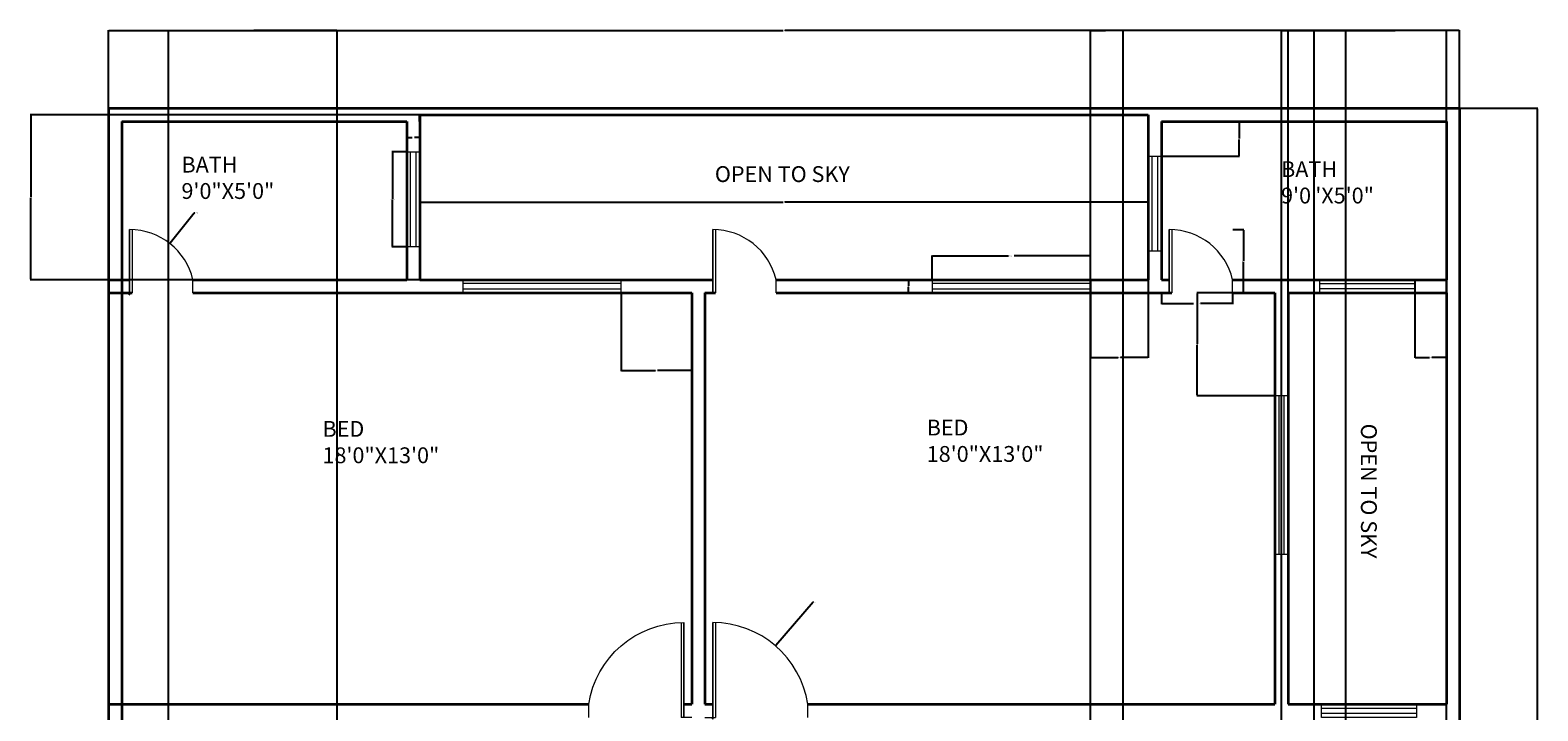
# Model space of a CAD drawing. Units: inches. Extents: x 40921 to 41493, y 89872 to 90511.
# Tile 4 of 4: x 40921 to 41493, y 90253 to 90511. Entities that reach past the tile are written whole.
import ezdxf

# ---------------------------------------------------------------- set-up
doc = ezdxf.new("R2010")
doc.units = ezdxf.units.IN
doc.header["$MEASUREMENT"] = 0
for name, color, linetype, lineweight in [('A-ANNO-DIMS', 2, 'Continuous', 18), ('A-AREA-IDEN', 7, 'Continuous', 18), ('A-DOOR', 3, 'Continuous', 20), ('A-GLAZ', 4, 'Continuous', 18), ('A-WALL', 7, 'Continuous', 35)]:
    doc.layers.add(name, color=color, linetype=linetype, lineweight=lineweight)
doc.styles.get("Standard").update_dxf_attribs({"font": 'arial.ttf'})
doc.dimstyles.get("Standard").update_dxf_attribs({"dimtxt": 0.18, "dimasz": 0.18, "dimexe": 0.18, "dimexo": 0.0625, "dimgap": 0.09, "dimtad": 0, "dimtih": 1, "dimtoh": 1, "dimdec": 4, "dimzin": 0, "dimdsep": 46, "dimtxsty": 'Standard', "dimcen": 0.09, "dimadec": 0, "dimazin": 0, "dimtfac": 1, "dimtdec": 4, "dimtofl": 0, "dimtmove": 0, "dimatfit": 3, "dimfxl": 1, "dimtolj": 1, "dimtzin": 0, "dimarcsym": 0})

# ---------------------------------------------------------------- blocks, each defined once
blk = doc.blocks.new('DOOR-SWING-24IN')
for p, q in [((3, 0), (3, 24)), ((3, 24), (3, 0)), ((4, 24), (4, 0)), ((27, 0), (27, 5)), ((0, 0), (3, 0)), ((3, 0), (4, 0))]:
    blk.add_line(p, q)
blk.add_arc((3, -0.66), 24.66, 13.265, 90)
blk = doc.blocks.new('DOOR-SWING-36IN')
for p, q in [((3, 0), (3, 36)), ((3, 36), (3, 0)), ((4, 36), (4, 0)), ((39, 0), (39, 5)), ((0, 0), (3, 0)), ((3, 0), (4, 0))]:
    blk.add_line(p, q)
blk.add_arc((3, -0.4), 36.4, 8.5358, 90)
blk = doc.blocks.new('WIN-36IN')
for p, q in [((0, 36), (5, 36)), ((0, 0), (0, 36)), ((1.5, 0), (1.5, 36)), ((3.5, 36), (3.5, 0)), ((5, 36), (5, 0)), ((5, 0), (0, 0))]:
    blk.add_line(p, q)
blk = doc.blocks.new('WIN-60IN')
for p, q in [((0, 5), (0, 0)), ((60, 5), (0, 5)), ((60, 3.5), (0, 3.5)), ((0, 1.5), (60, 1.5)), ((60, 0), (60, 5)), ((0, 0), (60, 0))]:
    blk.add_line(p, q)
blk = doc.blocks.new('*D7')
at = {"layer": 'A-ANNO-DIMS', "color": 0, "lineweight": -2, "transparency": 16777216}
for p, q in [((41064.09, 90465.09), (41058.57, 90465.09)), ((41058.75, 90464.91), (41058.75, 90447.27)), ((41058.75, 90429.27), (41058.75, 90446.9)), ((41064.09, 90429.09), (41058.57, 90429.09))]:
    blk.add_line(p, q, dxfattribs=at)
at = {"layer": 'A-ANNO-DIMS', "color": 0, "transparency": 16777216}
for points in [[(41058.72, 90464.91), (41058.78, 90464.91), (41058.75, 90465.09)], [(41058.72, 90429.27), (41058.78, 90429.27), (41058.75, 90429.09)]]:
    blk.add_solid(points, dxfattribs=at)
at = {"layer": 'Defpoints', "color": 0, "transparency": 16777216}
for p in [(41058.75, 90465.09), (41064.15, 90465.09), (41064.15, 90429.09)]:
    blk.add_point(p, dxfattribs=at)
at = {"layer": 'A-ANNO-DIMS', "color": 0, "transparency": 16777216, "insert": (41058.75, 90447.09), "char_height": 0.18, "attachment_point": 5}
blk.add_mtext('\\A1;WINDOW 36 TYP.', dxfattribs=at)
blk = doc.blocks.new('*D8')
at = {"layer": 'A-ANNO-DIMS', "color": 0, "lineweight": -2, "transparency": 16777216}
for p, q in [((41064.15, 90465.15), (41064.15, 90470.67)), ((41064.33, 90470.49), (41066.19, 90470.49)), ((41068.97, 90470.49), (41067.11, 90470.49)), ((41069.15, 90465.15), (41069.15, 90470.67))]:
    blk.add_line(p, q, dxfattribs=at)
at = {"layer": 'A-ANNO-DIMS', "color": 0, "transparency": 16777216}
for points in [[(41064.33, 90470.52), (41064.33, 90470.46), (41064.15, 90470.49)], [(41068.97, 90470.52), (41068.97, 90470.46), (41069.15, 90470.49)]]:
    blk.add_solid(points, dxfattribs=at)
at = {"layer": 'Defpoints', "color": 0, "transparency": 16777216}
for p in [(41069.15, 90470.49), (41064.15, 90465.09), (41069.15, 90465.09)]:
    blk.add_point(p, dxfattribs=at)
at = {"layer": 'A-ANNO-DIMS', "color": 0, "transparency": 16777216, "insert": (41066.65, 90470.49), "char_height": 0.18, "attachment_point": 5}
blk.add_mtext('\\A1;5 TYP.', dxfattribs=at)
blk = doc.blocks.new('*D9')
at = {"layer": 'A-ANNO-DIMS', "color": 0, "lineweight": -2, "transparency": 16777216}
for p, q in [((41263.29, 90416.69), (41263.29, 90425.81)), ((41263.47, 90425.63), (41292.18, 90425.63)), ((41323.11, 90425.63), (41294.41, 90425.63)), ((41323.29, 90416.69), (41323.29, 90425.81))]:
    blk.add_line(p, q, dxfattribs=at)
at = {"layer": 'A-ANNO-DIMS', "color": 0, "transparency": 16777216}
for points in [[(41263.47, 90425.66), (41263.47, 90425.6), (41263.29, 90425.63)], [(41323.11, 90425.66), (41323.11, 90425.6), (41323.29, 90425.63)]]:
    blk.add_solid(points, dxfattribs=at)
at = {"layer": 'Defpoints', "color": 0, "transparency": 16777216}
for p in [(41263.29, 90425.63), (41263.29, 90416.63), (41323.29, 90416.63)]:
    blk.add_point(p, dxfattribs=at)
at = {"layer": 'A-ANNO-DIMS', "color": 0, "transparency": 16777216, "insert": (41293.29, 90425.63), "char_height": 0.18, "attachment_point": 5}
blk.add_mtext('\\A1;WINDOW 60 TYP.', dxfattribs=at)
blk = doc.blocks.new('*D10')
at = {"layer": 'A-ANNO-DIMS', "color": 0, "lineweight": -2, "transparency": 16777216}
for p, q in [((41263.23, 90416.63), (41254.11, 90416.63)), ((41254.29, 90416.45), (41254.29, 90414.31)), ((41263.23, 90411.63), (41254.11, 90411.63)), ((41254.29, 90411.81), (41254.29, 90413.95))]:
    blk.add_line(p, q, dxfattribs=at)
at = {"layer": 'A-ANNO-DIMS', "color": 0, "transparency": 16777216}
for points in [[(41254.26, 90416.45), (41254.32, 90416.45), (41254.29, 90416.63)], [(41254.26, 90411.81), (41254.32, 90411.81), (41254.29, 90411.63)]]:
    blk.add_solid(points, dxfattribs=at)
at = {"layer": 'Defpoints', "color": 0, "transparency": 16777216}
for p in [(41263.29, 90416.63), (41254.29, 90411.63), (41263.29, 90411.63)]:
    blk.add_point(p, dxfattribs=at)
at = {"layer": 'A-ANNO-DIMS', "color": 0, "transparency": 16777216, "insert": (41254.29, 90414.13), "char_height": 0.18, "attachment_point": 5}
blk.add_mtext('\\A1;5 TYP.', dxfattribs=at)
blk = doc.blocks.new('*D13')
at = {"layer": 'A-ANNO-DIMS', "color": 0, "lineweight": -2, "transparency": 16777216}
for p, q in [((41350.15, 90411.57), (41350.15, 90407.4)), ((41377.15, 90411.57), (41377.15, 90407.4)), ((41350.33, 90407.58), (41362.34, 90407.58)), ((41376.97, 90407.58), (41364.96, 90407.58))]:
    blk.add_line(p, q, dxfattribs=at)
at = {"layer": 'A-ANNO-DIMS', "color": 0, "transparency": 16777216}
for points in [[(41350.33, 90407.61), (41350.33, 90407.55), (41350.15, 90407.58)], [(41376.97, 90407.61), (41376.97, 90407.55), (41377.15, 90407.58)]]:
    blk.add_solid(points, dxfattribs=at)
at = {"layer": 'Defpoints', "color": 0, "transparency": 16777216}
for p in [(41350.15, 90411.63), (41377.15, 90411.63), (41377.15, 90407.58)]:
    blk.add_point(p, dxfattribs=at)
at = {"layer": 'A-ANNO-DIMS', "color": 0, "transparency": 16777216, "insert": (41363.65, 90407.58), "char_height": 0.18, "attachment_point": 5}
blk.add_mtext('\\A1;BATH DOOR 27 TYP.', dxfattribs=at)
blk = doc.blocks.new('*D14')
at = {"layer": 'A-ANNO-DIMS', "color": 0, "lineweight": -2, "transparency": 16777216}
for p, q in [((41377.21, 90435.63), (41381.38, 90435.63)), ((41381.2, 90435.45), (41381.2, 90423.81)), ((41381.2, 90411.81), (41381.2, 90423.45)), ((41377.21, 90411.63), (41381.38, 90411.63))]:
    blk.add_line(p, q, dxfattribs=at)
at = {"layer": 'A-ANNO-DIMS', "color": 0, "transparency": 16777216}
for points in [[(41381.17, 90435.45), (41381.23, 90435.45), (41381.2, 90435.63)], [(41381.17, 90411.81), (41381.23, 90411.81), (41381.2, 90411.63)]]:
    blk.add_solid(points, dxfattribs=at)
at = {"layer": 'Defpoints', "color": 0, "transparency": 16777216}
for p in [(41377.15, 90435.63), (41381.2, 90435.63), (41377.15, 90411.63)]:
    blk.add_point(p, dxfattribs=at)
at = {"layer": 'A-ANNO-DIMS', "color": 0, "transparency": 16777216, "insert": (41381.2, 90423.63), "char_height": 0.18, "attachment_point": 5}
blk.add_mtext('\\A1;24 TYP.', dxfattribs=at)
blk = doc.blocks.new('*D19')
at = {"layer": 'A-ANNO-DIMS', "color": 0, "lineweight": -2, "transparency": 16777216}
for p, q in [((40951.15, 90481.69), (40951.15, 90511.26)), ((40951.33, 90511.08), (41206.86, 90511.08)), ((41462.97, 90511.08), (41207.44, 90511.08)), ((41463.15, 90481.69), (41463.15, 90511.26))]:
    blk.add_line(p, q, dxfattribs=at)
at = {"layer": 'A-ANNO-DIMS', "color": 0, "transparency": 16777216}
for points in [[(40951.33, 90511.11), (40951.33, 90511.05), (40951.15, 90511.08)], [(41462.97, 90511.11), (41462.97, 90511.05), (41463.15, 90511.08)]]:
    blk.add_solid(points, dxfattribs=at)
at = {"layer": 'Defpoints', "color": 0, "transparency": 16777216}
for p in [(41463.15, 90511.08), (40951.15, 90481.63), (41463.15, 90481.63)]:
    blk.add_point(p, dxfattribs=at)
at = {"layer": 'A-ANNO-DIMS', "color": 0, "transparency": 16777216, "insert": (41207.15, 90511.08), "char_height": 0.18, "attachment_point": 5}
blk.add_mtext('\\A1;512', dxfattribs=at)
blk = doc.blocks.new('*D20')
at = {"layer": 'A-ANNO-DIMS', "color": 0, "lineweight": -2, "transparency": 16777216}
for p, q in [((41463.21, 90481.63), (41492.78, 90481.63)), ((41492.6, 90481.45), (41492.6, 90191.81)), ((41492.6, 89901.81), (41492.6, 90191.45)), ((41463.21, 89901.63), (41492.78, 89901.63))]:
    blk.add_line(p, q, dxfattribs=at)
at = {"layer": 'A-ANNO-DIMS', "color": 0, "transparency": 16777216}
for points in [[(41492.57, 90481.45), (41492.63, 90481.45), (41492.6, 90481.63)], [(41492.57, 89901.81), (41492.63, 89901.81), (41492.6, 89901.63)]]:
    blk.add_solid(points, dxfattribs=at)
at = {"layer": 'Defpoints', "color": 0, "transparency": 16777216}
for p in [(41463.15, 90481.63), (41492.6, 90481.63), (41463.15, 89901.63)]:
    blk.add_point(p, dxfattribs=at)
at = {"layer": 'A-ANNO-DIMS', "color": 0, "transparency": 16777216, "insert": (41492.6, 90191.63), "char_height": 0.18, "attachment_point": 5}
blk.add_mtext('\\A1;580', dxfattribs=at)
blk = doc.blocks.new('*D21')
at = {"layer": 'A-ANNO-DIMS', "color": 0, "lineweight": -2, "transparency": 16777216}
for p, q in [((41069.15, 90416.69), (41069.15, 90446.26)), ((41069.33, 90446.08), (41206.86, 90446.08)), ((41344.97, 90446.08), (41207.44, 90446.08)), ((41345.15, 90416.69), (41345.15, 90446.26))]:
    blk.add_line(p, q, dxfattribs=at)
at = {"layer": 'A-ANNO-DIMS', "color": 0, "transparency": 16777216}
for points in [[(41069.33, 90446.11), (41069.33, 90446.05), (41069.15, 90446.08)], [(41344.97, 90446.11), (41344.97, 90446.05), (41345.15, 90446.08)]]:
    blk.add_solid(points, dxfattribs=at)
at = {"layer": 'Defpoints', "color": 0, "transparency": 16777216}
for p in [(41345.15, 90446.08), (41069.15, 90416.63), (41345.15, 90416.63)]:
    blk.add_point(p, dxfattribs=at)
at = {"layer": 'A-ANNO-DIMS', "color": 0, "transparency": 16777216, "insert": (41207.15, 90446.08), "char_height": 0.18, "attachment_point": 5}
blk.add_mtext('\\A1;276', dxfattribs=at)
blk = doc.blocks.new('*D22')
at = {"layer": 'A-ANNO-DIMS', "color": 0, "lineweight": -2, "transparency": 16777216}
for p, q in [((41069.09, 90479.13), (40921.52, 90479.13)), ((40921.7, 90478.95), (40921.7, 90448.06)), ((40921.7, 90416.81), (40921.7, 90447.7)), ((41069.09, 90416.63), (40921.52, 90416.63))]:
    blk.add_line(p, q, dxfattribs=at)
at = {"layer": 'A-ANNO-DIMS', "color": 0, "transparency": 16777216}
for points in [[(40921.67, 90478.95), (40921.73, 90478.95), (40921.7, 90479.13)], [(40921.67, 90416.81), (40921.73, 90416.81), (40921.7, 90416.63)]]:
    blk.add_solid(points, dxfattribs=at)
at = {"layer": 'Defpoints', "color": 0, "transparency": 16777216}
for p in [(41069.15, 90479.13), (40921.7, 90416.63), (41069.15, 90416.63)]:
    blk.add_point(p, dxfattribs=at)
at = {"layer": 'A-ANNO-DIMS', "color": 0, "transparency": 16777216, "insert": (40921.7, 90447.88), "char_height": 0.18, "attachment_point": 5}
blk.add_mtext('\\A1;62.5', dxfattribs=at)
blk = doc.blocks.new('*D23')
at = {"layer": 'A-ANNO-DIMS', "color": 0, "lineweight": -2, "transparency": 16777216}
for p, q in [((41398.15, 90255.69), (41398.15, 90511.26)), ((41398.33, 90511.08), (41427.93, 90511.08)), ((41457.97, 90511.08), (41428.37, 90511.08)), ((41458.15, 90255.69), (41458.15, 90511.26))]:
    blk.add_line(p, q, dxfattribs=at)
at = {"layer": 'A-ANNO-DIMS', "color": 0, "transparency": 16777216}
for points in [[(41398.33, 90511.11), (41398.33, 90511.05), (41398.15, 90511.08)], [(41457.97, 90511.11), (41457.97, 90511.05), (41458.15, 90511.08)]]:
    blk.add_solid(points, dxfattribs=at)
at = {"layer": 'Defpoints', "color": 0, "transparency": 16777216}
for p in [(41458.15, 90511.08), (41398.15, 90255.63), (41458.15, 90255.63)]:
    blk.add_point(p, dxfattribs=at)
at = {"layer": 'A-ANNO-DIMS', "color": 0, "transparency": 16777216, "insert": (41428.15, 90511.08), "char_height": 0.18, "attachment_point": 5}
blk.add_mtext('\\A1;60', dxfattribs=at)
blk = doc.blocks.new('*D25')
at = {"layer": 'A-ANNO-DIMS', "color": 0, "lineweight": -2, "transparency": 16777216}
for p, q in [((40973.9, 90106.69), (40973.9, 90511.26)), ((40974.08, 90511.08), (41005.48, 90511.08)), ((41037.63, 90511.08), (41006.23, 90511.08)), ((41037.81, 90106.69), (41037.81, 90511.26))]:
    blk.add_line(p, q, dxfattribs=at)
at = {"layer": 'A-ANNO-DIMS', "color": 0, "transparency": 16777216}
for points in [[(40974.08, 90511.11), (40974.08, 90511.05), (40973.9, 90511.08)], [(41037.63, 90511.11), (41037.63, 90511.05), (41037.81, 90511.08)]]:
    blk.add_solid(points, dxfattribs=at)
at = {"layer": 'Defpoints', "color": 0, "transparency": 16777216}
for p in [(41037.81, 90511.08), (40973.9, 90106.63), (41037.81, 90106.63)]:
    blk.add_point(p, dxfattribs=at)
at = {"layer": 'A-ANNO-DIMS', "color": 0, "transparency": 16777216, "insert": (41005.85, 90511.08), "char_height": 0.18, "attachment_point": 5}
blk.add_mtext('\\A1;63.91', dxfattribs=at)
blk = doc.blocks.new('*D31')
at = {"layer": 'A-ANNO-DIMS', "color": 0, "lineweight": -2, "transparency": 16777216}
for p, q in [((41420.03, 89906.69), (41420.03, 90511.26)), ((41420.21, 90511.08), (41438.7, 90511.08)), ((41457.97, 90511.08), (41439.48, 90511.08)), ((41458.15, 89906.69), (41458.15, 90511.26))]:
    blk.add_line(p, q, dxfattribs=at)
at = {"layer": 'A-ANNO-DIMS', "color": 0, "transparency": 16777216}
for points in [[(41420.21, 90511.11), (41420.21, 90511.05), (41420.03, 90511.08)], [(41457.97, 90511.11), (41457.97, 90511.05), (41458.15, 90511.08)]]:
    blk.add_solid(points, dxfattribs=at)
at = {"layer": 'Defpoints', "color": 0, "transparency": 16777216}
for p in [(41458.15, 90511.08), (41420.03, 89906.63), (41458.15, 89906.63)]:
    blk.add_point(p, dxfattribs=at)
at = {"layer": 'A-ANNO-DIMS', "color": 0, "transparency": 16777216, "insert": (41439.09, 90511.08), "char_height": 0.18, "attachment_point": 5}
blk.add_mtext('\\A1;38.12', dxfattribs=at)
blk = doc.blocks.new('*D32')
at = {"layer": 'A-ANNO-DIMS', "color": 0, "lineweight": -2, "transparency": 16777216}
for p, q in [((41323.33, 89906.69), (41323.33, 90511.26)), ((41323.51, 90511.08), (41329.01, 90511.08)), ((41335.42, 90511.08), (41329.92, 90511.08)), ((41335.6, 89906.69), (41335.6, 90511.26))]:
    blk.add_line(p, q, dxfattribs=at)
at = {"layer": 'A-ANNO-DIMS', "color": 0, "transparency": 16777216}
for points in [[(41323.51, 90511.11), (41323.51, 90511.05), (41323.33, 90511.08)], [(41335.42, 90511.11), (41335.42, 90511.05), (41335.6, 90511.08)]]:
    blk.add_solid(points, dxfattribs=at)
at = {"layer": 'Defpoints', "color": 0, "transparency": 16777216}
for p in [(41335.6, 90511.08), (41323.33, 89906.63), (41335.6, 89906.63)]:
    blk.add_point(p, dxfattribs=at)
at = {"layer": 'A-ANNO-DIMS', "color": 0, "transparency": 16777216, "insert": (41329.46, 90511.08), "char_height": 0.18, "attachment_point": 5}
blk.add_mtext('\\A1;12.272', dxfattribs=at)
blk = doc.blocks.new('*D33')
at = {"layer": 'A-ANNO-DIMS', "color": 0, "lineweight": -2, "transparency": 16777216}
for p, q in [((41395.6, 89906.69), (41395.6, 90511.26)), ((41395.78, 90511.08), (41401.36, 90511.08)), ((41407.85, 90511.08), (41402.27, 90511.08)), ((41408.03, 89906.69), (41408.03, 90511.26))]:
    blk.add_line(p, q, dxfattribs=at)
at = {"layer": 'A-ANNO-DIMS', "color": 0, "transparency": 16777216}
for points in [[(41395.78, 90511.11), (41395.78, 90511.05), (41395.6, 90511.08)], [(41407.85, 90511.11), (41407.85, 90511.05), (41408.03, 90511.08)]]:
    blk.add_solid(points, dxfattribs=at)
at = {"layer": 'Defpoints', "color": 0, "transparency": 16777216}
for p in [(41408.03, 90511.08), (41395.6, 89906.63), (41408.03, 89906.63)]:
    blk.add_point(p, dxfattribs=at)
at = {"layer": 'A-ANNO-DIMS', "color": 0, "transparency": 16777216, "insert": (41401.81, 90511.08), "char_height": 0.18, "attachment_point": 5}
blk.add_mtext('\\A1;12.429', dxfattribs=at)
blk = doc.blocks.new('*D36')
at = {"layer": 'A-ANNO-DIMS', "color": 0, "lineweight": -2, "transparency": 16777216}
for p, q in [((41145.4, 90411.57), (41145.4, 90382)), ((41172.15, 90411.57), (41172.15, 90382)), ((41145.58, 90382.18), (41158.38, 90382.18)), ((41171.97, 90382.18), (41159.17, 90382.18))]:
    blk.add_line(p, q, dxfattribs=at)
at = {"layer": 'A-ANNO-DIMS', "color": 0, "transparency": 16777216}
for points in [[(41145.58, 90382.21), (41145.58, 90382.15), (41145.4, 90382.18)], [(41171.97, 90382.21), (41171.97, 90382.15), (41172.15, 90382.18)]]:
    blk.add_solid(points, dxfattribs=at)
at = {"layer": 'Defpoints', "color": 0, "transparency": 16777216}
for p in [(41145.4, 90411.63), (41172.15, 90411.63), (41145.4, 90382.18)]:
    blk.add_point(p, dxfattribs=at)
at = {"layer": 'A-ANNO-DIMS', "color": 0, "transparency": 16777216, "insert": (41158.77, 90382.18), "char_height": 0.18, "attachment_point": 5}
blk.add_mtext('\\A1;26.75', dxfattribs=at)
blk = doc.blocks.new('*D37')
at = {"layer": 'A-ANNO-DIMS', "color": 0, "lineweight": -2, "transparency": 16777216}
for p, q in [((41323.29, 90416.57), (41323.29, 90387)), ((41345.15, 90416.57), (41345.15, 90387)), ((41323.47, 90387.18), (41333.76, 90387.18)), ((41344.97, 90387.18), (41334.69, 90387.18))]:
    blk.add_line(p, q, dxfattribs=at)
at = {"layer": 'A-ANNO-DIMS', "color": 0, "transparency": 16777216}
for points in [[(41323.47, 90387.21), (41323.47, 90387.15), (41323.29, 90387.18)], [(41344.97, 90387.21), (41344.97, 90387.15), (41345.15, 90387.18)]]:
    blk.add_solid(points, dxfattribs=at)
at = {"layer": 'Defpoints', "color": 0, "transparency": 16777216}
for p in [(41323.29, 90416.63), (41345.15, 90416.63), (41323.29, 90387.18)]:
    blk.add_point(p, dxfattribs=at)
at = {"layer": 'A-ANNO-DIMS', "color": 0, "transparency": 16777216, "insert": (41334.22, 90387.18), "char_height": 0.18, "attachment_point": 5}
blk.add_mtext('\\A1;21.857', dxfattribs=at)
blk = doc.blocks.new('*D38')
at = {"layer": 'A-ANNO-DIMS', "color": 0, "lineweight": -2, "transparency": 16777216}
for p, q in [((41393.09, 90411.63), (41363.52, 90411.63)), ((41363.7, 90411.45), (41363.7, 90392.3)), ((41363.7, 90372.79), (41363.7, 90391.94)), ((41393.09, 90372.61), (41363.52, 90372.61))]:
    blk.add_line(p, q, dxfattribs=at)
at = {"layer": 'A-ANNO-DIMS', "color": 0, "transparency": 16777216}
for points in [[(41363.67, 90411.45), (41363.73, 90411.45), (41363.7, 90411.63)], [(41363.67, 90372.79), (41363.73, 90372.79), (41363.7, 90372.61)]]:
    blk.add_solid(points, dxfattribs=at)
at = {"layer": 'Defpoints', "color": 0, "transparency": 16777216}
for p in [(41363.7, 90411.63), (41393.15, 90411.63), (41393.15, 90372.61)]:
    blk.add_point(p, dxfattribs=at)
at = {"layer": 'A-ANNO-DIMS', "color": 0, "transparency": 16777216, "insert": (41363.7, 90392.12), "char_height": 0.18, "attachment_point": 5}
blk.add_mtext('\\A1;39.02', dxfattribs=at)
blk = doc.blocks.new('*D39')
at = {"layer": 'A-ANNO-DIMS', "color": 0, "lineweight": -2, "transparency": 16777216}
for p, q in [((41446.17, 90416.57), (41446.17, 90387)), ((41458.15, 90416.57), (41458.15, 90387)), ((41446.35, 90387.18), (41451.7, 90387.18)), ((41457.97, 90387.18), (41452.61, 90387.18))]:
    blk.add_line(p, q, dxfattribs=at)
at = {"layer": 'A-ANNO-DIMS', "color": 0, "transparency": 16777216}
for points in [[(41446.35, 90387.21), (41446.35, 90387.15), (41446.17, 90387.18)], [(41457.97, 90387.21), (41457.97, 90387.15), (41458.15, 90387.18)]]:
    blk.add_solid(points, dxfattribs=at)
at = {"layer": 'Defpoints', "color": 0, "transparency": 16777216}
for p in [(41446.17, 90416.63), (41458.15, 90416.63), (41446.17, 90387.18)]:
    blk.add_point(p, dxfattribs=at)
at = {"layer": 'A-ANNO-DIMS', "color": 0, "transparency": 16777216, "insert": (41452.16, 90387.18), "char_height": 0.18, "attachment_point": 5}
blk.add_mtext('\\A1;11.983', dxfattribs=at)
blk = doc.blocks.new('*D45')
at = {"layer": 'A-ANNO-DIMS', "color": 0, "lineweight": -2, "transparency": 16777216}
for p, q in [((41350.21, 90476.63), (41379.78, 90476.63)), ((41379.6, 90476.45), (41379.6, 90470.21)), ((41379.6, 90463.61), (41379.6, 90469.85)), ((41350.21, 90463.43), (41379.78, 90463.43))]:
    blk.add_line(p, q, dxfattribs=at)
at = {"layer": 'A-ANNO-DIMS', "color": 0, "transparency": 16777216}
for points in [[(41379.57, 90476.45), (41379.63, 90476.45), (41379.6, 90476.63)], [(41379.57, 90463.61), (41379.63, 90463.61), (41379.6, 90463.43)]]:
    blk.add_solid(points, dxfattribs=at)
at = {"layer": 'Defpoints', "color": 0, "transparency": 16777216}
for p in [(41350.15, 90476.63), (41350.15, 90463.43), (41379.6, 90463.43)]:
    blk.add_point(p, dxfattribs=at)
at = {"layer": 'A-ANNO-DIMS', "color": 0, "transparency": 16777216, "insert": (41379.6, 90470.03), "char_height": 0.18, "attachment_point": 5}
blk.add_mtext('\\A1;13.197', dxfattribs=at)
blk = doc.blocks.new('*D46')
at = {"layer": 'A-ANNO-DIMS', "color": 0, "lineweight": -2, "transparency": 16777216}
for p, q in [((41218.16, 90294.36), (41204.02, 90277.95)), ((41218.34, 90294.36), (41218.16, 90294.36)), ((41180.06, 90250.23), (41180.24, 90250.23)), ((41180.15, 90250.14), (41180.15, 90250.32))]:
    blk.add_line(p, q, dxfattribs=at)
at = {"layer": 'A-ANNO-DIMS', "color": 0, "transparency": 16777216}
blk.add_solid([(41204, 90277.97), (41204.04, 90277.93), (41203.9, 90277.81)], dxfattribs=at)
at = {"layer": 'Defpoints', "color": 0, "transparency": 16777216}
for p in [(41203.9, 90277.81), (41180.15, 90250.23)]:
    blk.add_point(p, dxfattribs=at)
at = {"layer": 'A-ANNO-DIMS', "color": 0, "transparency": 16777216, "insert": (41218.94, 90294.36), "char_height": 0.18, "attachment_point": 5}
blk.add_mtext('\\A1;2X R36.4', dxfattribs=at)
blk = doc.blocks.new('*D47')
at = {"layer": 'A-ANNO-DIMS', "color": 0, "lineweight": -2, "transparency": 16777216}
for p, q in [((40983.64, 90441.91), (40974.57, 90430.45)), ((40983.82, 90441.91), (40983.64, 90441.91)), ((40959.06, 90410.97), (40959.24, 90410.97)), ((40959.15, 90410.88), (40959.15, 90411.06))]:
    blk.add_line(p, q, dxfattribs=at)
at = {"layer": 'A-ANNO-DIMS', "color": 0, "transparency": 16777216}
blk.add_solid([(40974.54, 90430.47), (40974.59, 90430.43), (40974.46, 90430.31)], dxfattribs=at)
at = {"layer": 'Defpoints', "color": 0, "transparency": 16777216}
for p in [(40974.46, 90430.31), (40959.15, 90410.97)]:
    blk.add_point(p, dxfattribs=at)
at = {"layer": 'A-ANNO-DIMS', "color": 0, "transparency": 16777216, "insert": (40984.49, 90441.91), "char_height": 0.18, "attachment_point": 5}
blk.add_mtext('\\A1;5X R24.66', dxfattribs=at)

msp = doc.modelspace()

# ---------------------------------------------------------------- linework, layer by layer
at = {"layer": 'A-GLAZ'}
for p, q in [((41064.1503, 90465.0876), (41064.1503, 90465.0876)), ((41446.167, 90416.6306), (41446.167, 90416.6306))]:
    msp.add_line(p, q, dxfattribs=at)
at = {"layer": 'A-WALL'}
for p, q in [((40951.1503, 90481.6306), (41463.1503, 90481.6306)), ((40951.1503, 90481.6306), (40951.1503, 89901.6306)), ((41069.1503, 90479.1306), (41069.1503, 90416.6306)), ((41069.1503, 90479.1306), (41069.1503, 90476.6306)), ((41069.1503, 90476.6306), (41069.1503, 90479.1306)), ((41069.1503, 90479.1306), (41345.1503, 90479.1306)), ((41345.1503, 90479.1306), (41345.1503, 90416.6306)), ((41463.1503, 90481.6306), (41463.1503, 89901.6306)), ((40956.1503, 90476.6306), (40956.1503, 90106.6306)), ((40956.1503, 90476.6306), (41064.1503, 90476.6306)), ((41064.1503, 90476.6306), (41064.1503, 90416.6306)), ((41350.1503, 90476.6306), (41350.1503, 90416.6306)), ((41350.1503, 90476.6306), (41458.1503, 90476.6306)), ((41458.1503, 90476.6306), (41458.1503, 90416.6306)), ((40951.1503, 90416.6306), (40959.1503, 90416.6306)), ((40983.1503, 90416.6306), (41064.1503, 90416.6306)), ((41069.1503, 90416.6306), (41180.1503, 90416.6306)), ((41204.1503, 90416.6306), (41345.1503, 90416.6306)), ((41350.1503, 90416.6306), (41353.1503, 90416.6306)), ((41377.1503, 90416.6306), (41458.1503, 90416.6306)), ((40951.1503, 90411.6306), (40960.1503, 90411.6306)), ((40983.1503, 90411.6306), (41172.1503, 90411.6306)), ((41172.1503, 90411.6306), (41172.1503, 90255.6306)), ((41177.1503, 90411.6306), (41177.1503, 90255.6306)), ((41177.1503, 90411.6306), (41181.1503, 90411.6306)), ((41204.1503, 90411.6306), (41354.1503, 90411.6306)), ((41377.1503, 90411.6306), (41393.1503, 90411.6306)), ((41393.1503, 90411.6306), (41393.1503, 90255.6306)), ((41398.1503, 90411.6306), (41398.1503, 90255.6306)), ((41398.1503, 90411.6306), (41458.1503, 90411.6306)), ((41458.1503, 90411.6306), (41458.1503, 90255.6306)), ((40951.1503, 90255.6306), (41133.1503, 90255.6306)), ((41169.1503, 90255.6306), (41172.1503, 90255.6306)), ((41177.1503, 90255.6306), (41180.1503, 90255.6306)), ((41216.1503, 90255.6306), (41393.1503, 90255.6306)), ((41398.1503, 90255.6306), (41458.1503, 90255.6306))]:
    msp.add_line(p, q, dxfattribs=at)

# ---------------------------------------------------------------- block references
at = {"layer": 'A-DOOR'}
for name, p in [('DOOR-SWING-24IN', (40956.15, 90411.631)), ('DOOR-SWING-24IN', (41177.15, 90411.631)), ('DOOR-SWING-24IN', (41350.15, 90411.631)), ('DOOR-SWING-36IN', (41177.15, 90250.631))]:
    msp.add_blockref(name, p, dxfattribs=at)
at = {"layer": 'A-DOOR', "extrusion": (0, 0, -1), "zscale": -1}
msp.add_blockref('DOOR-SWING-36IN', (-41172.1506, 90250.631), dxfattribs=at)
at = {"layer": 'A-GLAZ'}
for name, p in [('WIN-36IN', (41064.15, 90429.088)), ('WIN-36IN', (41345.15, 90427.434)), ('WIN-60IN', (41085.398, 90411.631))]:
    msp.add_blockref(name, p, dxfattribs=at)
for name, p, rotation in [('WIN-60IN', (41323.2934, 90416.6303), 180), ('WIN-36IN', (41446.1666, 90411.6303), 90.00000000000003), ('WIN-60IN', (41393.1507, 90372.6125), 269.9999999999988), ('WIN-36IN', (41446.8101, 90250.6303), 89.99999999999685)]:
    msp.add_blockref(name, p, dxfattribs=dict(at, rotation=rotation))

# ---------------------------------------------------------------- texts
at = {"layer": 'A-AREA-IDEN', "char_height": 6, "attachment_point": 1}
for s, width, insert in [('BATH\\P9\'0"X5\'0"', 65.892116, (40978.8038, 90463.2623)), ('BATH\\P9\'0"X5\'0"', 65.892116, (41395.5067, 90461.5403)), ('OPEN TO SKY', 111.644025, (41180.9345, 90459.6692)), ('BED\\P18\'0"X13\'0"', 70.467307, (41032.2403, 90363.0531)), ('BED\\P18\'0"X13\'0"', 70.467307, (41261.2097, 90363.5572))]:
    msp.add_mtext_dynamic_manual_height_columns(s, width=width, gutter_width=1, heights=[0], dxfattribs=dict(at, insert=insert))
at = {"layer": 'A-AREA-IDEN', "insert": (41431.7814, 90362.0468), "char_height": 6, "attachment_point": 1, "rotation": 270}
msp.add_mtext_dynamic_manual_height_columns('OPEN TO SKY', width=111.644025, gutter_width=1, heights=[0], dxfattribs=at)

# ---------------------------------------------------------------- dimensions: what is measured, and where the dimension line sits
at = {"layer": 'A-ANNO-DIMS'}
for base, p1, p2, override, picture, middle in [((41463.1503, 90511.0806), (40951.1503, 90481.6306), (41463.1503, 90481.6306), {"dimdec": 0, "dimlfac": 1, "dimrnd": 0, "dimzin": 0, "dimdsep": 46, "dimlunit": 2}, '*D19', (41207.1503, 90511.0806)), ((41037.8072, 90511.0806), (40973.8989, 90106.6306), (41037.8072, 90106.6306), {"dimdec": 2, "dimlfac": 1, "dimrnd": 0, "dimzin": 0, "dimdsep": 46, "dimlunit": 2}, '*D25', (41005.8531, 90511.0806)), ((41335.5998, 90511.0806), (41323.3274, 89906.6306), (41335.5998, 89906.6306), {"dimdec": 3, "dimlfac": 1, "dimrnd": 0, "dimzin": 0, "dimdsep": 46, "dimlunit": 2}, '*D32', (41329.4636, 90511.0806)), ((41408.028255, 90511.080628), (41395.599751, 89906.630628), (41408.028255, 89906.630628), {"dimdec": 3, "dimlfac": 1, "dimrnd": 0, "dimzin": 0, "dimdsep": 46, "dimlunit": 2}, '*D33', (41401.814003, 90511.080628)), ((41458.1503, 90511.0806), (41398.1503, 90255.6306), (41458.1503, 90255.6306), {"dimdec": 0, "dimlfac": 1, "dimrnd": 0, "dimzin": 0, "dimdsep": 46, "dimlunit": 2}, '*D23', (41428.1503, 90511.0806)), ((41458.1503, 90511.0806), (41420.0283, 89906.6306), (41458.1503, 89906.6306), {"dimdec": 2, "dimlfac": 1, "dimrnd": 0, "dimzin": 0, "dimdsep": 46, "dimlunit": 2}, '*D31', (41439.0893, 90511.0806)), ((41345.1503, 90446.0806), (41069.1503, 90416.6306), (41345.1503, 90416.6306), {"dimdec": 0, "dimlfac": 1, "dimrnd": 0, "dimzin": 0, "dimdsep": 46, "dimlunit": 2}, '*D21', (41207.1503, 90446.0806))]:
    dim = msp.add_linear_dim(base=base, p1=p1, p2=p2, dimstyle='Standard', override=override, dxfattribs=at)
    dim.commit()
    dim.dimension.update_dxf_attribs({"geometry": picture, "text_midpoint": middle})
for base, p1, p2, angle, override, picture, middle in [((40921.7003, 90416.6306), (41069.1503, 90479.1306), (41069.1503, 90416.6306), 90, {"dimdec": 1, "dimlfac": 1, "dimrnd": 0, "dimzin": 0, "dimdsep": 46, "dimlunit": 2}, '*D22', (40921.7003, 90447.8806)), ((41492.6003, 90481.6306), (41463.1503, 89901.6306), (41463.1503, 90481.6306), 90, {"dimdec": 0, "dimlfac": 1, "dimrnd": 0, "dimzin": 0, "dimdsep": 46, "dimlunit": 2}, '*D20', (41492.6003, 90191.6306)), ((41379.6003, 90463.4336), (41350.1503, 90476.6306), (41350.1503, 90463.4336), 270, {"dimdec": 3, "dimlfac": 1, "dimrnd": 0, "dimzin": 0, "dimdsep": 46, "dimlunit": 2}, '*D45', (41379.6003, 90470.0321)), ((41323.2936, 90387.1806), (41345.1503, 90416.6306), (41323.2936, 90416.6306), 180, {"dimdec": 3, "dimlfac": 1, "dimrnd": 0, "dimzin": 0, "dimdsep": 46, "dimlunit": 2}, '*D37', (41334.222, 90387.1806)), ((41446.167, 90387.1806), (41458.1503, 90416.6306), (41446.167, 90416.6306), 180, {"dimdec": 3, "dimlfac": 1, "dimrnd": 0, "dimzin": 0, "dimdsep": 46, "dimlunit": 2}, '*D39', (41452.1587, 90387.1806)), ((41145.3978, 90382.1806), (41172.1503, 90411.6306), (41145.3978, 90411.6306), 180, {"dimdec": 2, "dimlfac": 1, "dimrnd": 0, "dimzin": 0, "dimdsep": 46, "dimlunit": 2}, '*D36', (41158.774, 90382.1806)), ((41363.7003, 90411.6306), (41393.1503, 90372.6128), (41393.1503, 90411.6306), 90, {"dimdec": 2, "dimlfac": 1, "dimrnd": 0, "dimzin": 0, "dimdsep": 46, "dimlunit": 2}, '*D38', (41363.7003, 90392.1217))]:
    dim = msp.add_linear_dim(base=base, p1=p1, p2=p2, angle=angle, dimstyle='Standard', override=override, dxfattribs=at)
    dim.commit()
    dim.dimension.update_dxf_attribs({"geometry": picture, "text_midpoint": middle})
for base, p1, p2, text, picture, middle in [((41069.1503, 90470.4876), (41064.1503, 90465.0876), (41069.1503, 90465.0876), '<> TYP.', '*D8', (41066.6503, 90470.4876)), ((41377.1503, 90407.5806), (41350.1503, 90411.6306), (41377.1503, 90411.6306), 'BATH DOOR <> TYP.', '*D13', (41363.6503, 90407.5806))]:
    dim = msp.add_linear_dim(base=base, p1=p1, p2=p2, text=text, dimstyle='Standard', override={"dimdec": 0, "dimlfac": 1, "dimrnd": 0, "dimzin": 0, "dimdsep": 46, "dimlunit": 2}, dxfattribs=at)
    dim.commit()
    dim.dimension.update_dxf_attribs({"geometry": picture, "text_midpoint": middle})
for base, p1, p2, angle, text, picture, middle in [((41058.7503, 90465.0876), (41064.1503, 90429.0876), (41064.1503, 90465.0876), 90, 'WINDOW <> TYP.', '*D7', (41058.7503, 90447.0876)), ((41381.2003, 90435.6306), (41377.1503, 90411.6306), (41377.1503, 90435.6306), 90, '<> TYP.', '*D14', (41381.2003, 90423.6306)), ((41263.2936, 90425.6306), (41323.2936, 90416.6306), (41263.2936, 90416.6306), 180, 'WINDOW <> TYP.', '*D9', (41293.2936, 90425.6306)), ((41254.2936, 90411.6306), (41263.2936, 90416.6306), (41263.2936, 90411.6306), 270, '<> TYP.', '*D10', (41254.2936, 90414.1306))]:
    dim = msp.add_linear_dim(base=base, p1=p1, p2=p2, angle=angle, text=text, dimstyle='Standard', override={"dimdec": 0, "dimlfac": 1, "dimrnd": 0, "dimzin": 0, "dimdsep": 46, "dimlunit": 2}, dxfattribs=at)
    dim.commit()
    dim.dimension.update_dxf_attribs({"geometry": picture, "text_midpoint": middle})
for center, mpoint, text, override, picture, middle in [((40959.1503, 90410.9727), (40974.4557, 90430.3056), '5X <>', {"dimdec": 2, "dimlfac": 1, "dimrnd": 0, "dimzin": 0, "dimdsep": 46, "dimlunit": 2}, '*D47', (40984.492, 90441.9053)), ((41180.1503, 90250.2274), (41203.9039, 90277.8129), '2X <>', {"dimdec": 1, "dimlfac": 1, "dimrnd": 0, "dimzin": 0, "dimdsep": 46, "dimlunit": 2}, '*D46', (41218.9406, 90294.3642))]:
    dim = msp.add_radius_dim(center=center, mpoint=mpoint, text=text, dimstyle='Standard', override=override, dxfattribs=at)
    dim.commit()
    dim.dimension.update_dxf_attribs({"geometry": picture, "text_midpoint": middle, "dimtype": 164})

doc.saveas('drawing.dxf')
